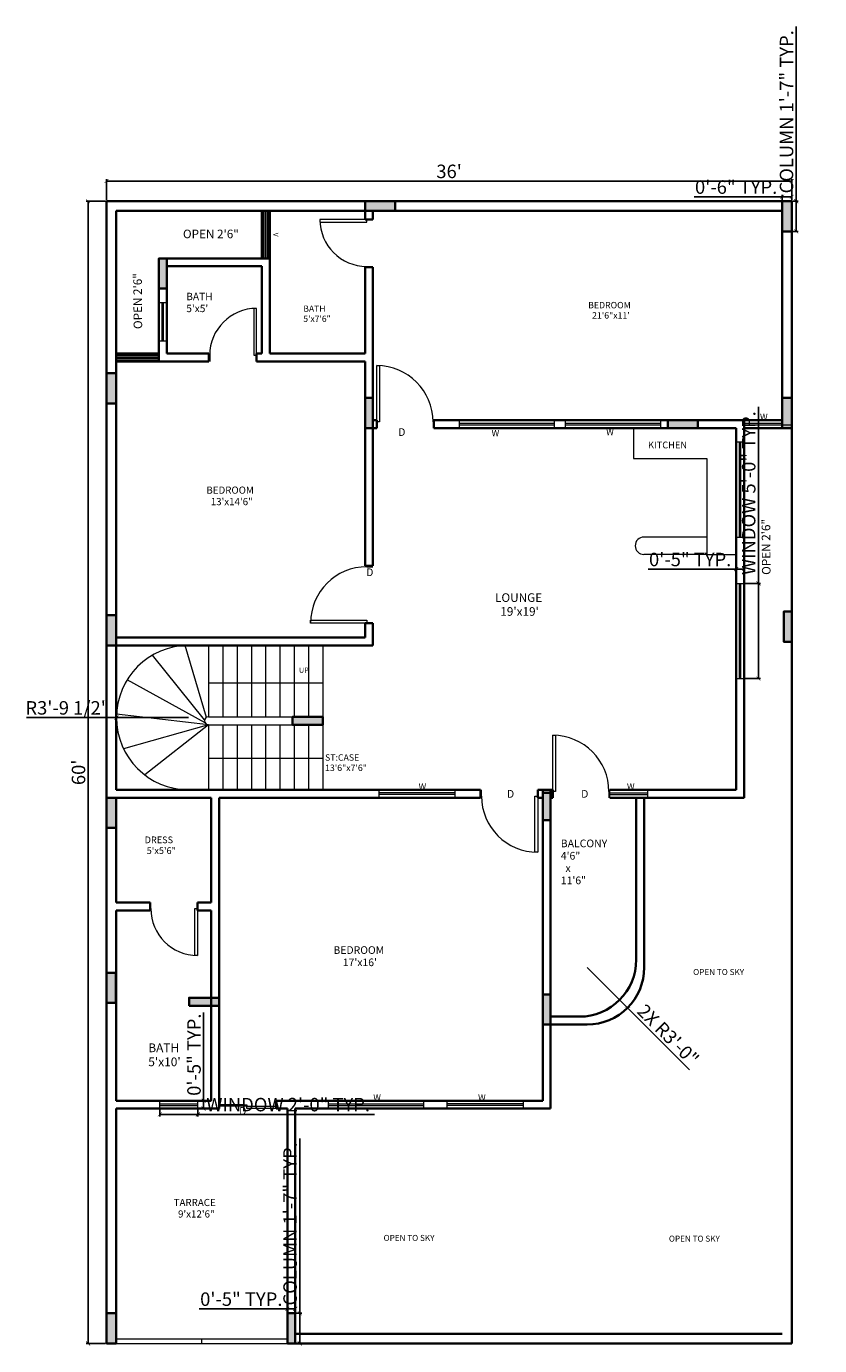
# Model space of a CAD drawing. Units: inches. Extents: x 3799 to 20199, y 1682 to 8087.
# Tile 23 of 30: x 13824 to 14325, y 7134 to 7966. Entities that reach past the tile are written whole.
import ezdxf

# ---------------------------------------------------------------- set-up
doc = ezdxf.new("R2010")
doc.units = ezdxf.units.IN
for name, color, linetype, lineweight in [('A-ANNO-DIMS', 2, 'Continuous', 18), ('A-ANNO-SYMB', 3, 'Continuous', 18), ('A-AREA-IDEN', 7, 'Continuous', 18), ('A-COLS', 251, 'Continuous', 35), ('A-DOOR', 3, 'Continuous', 18), ('A-FLOR-CASE', 32, 'Continuous', 18), ('A-FLOR-RAIL', 217, 'Continuous', 18), ('A-FLOR-STRS', 41, 'Continuous', 18), ('A-GLAZ', 152, 'Continuous', 18), ('A-WALL', 7, 'Continuous', 35)]:
    doc.layers.add(name, color=color, linetype=linetype, lineweight=lineweight)
doc.styles.get("Standard").update_dxf_attribs({"font": 'arial.ttf'})
doc.dimstyles.new('ISO-25', dxfattribs={"dimtxt": 8.5, "dimasz": 2.5, "dimexe": 1.25, "dimexo": 0.625, "dimtad": 1, "dimdec": 0, "dimlunit": 3, "dimtxsty": 'Standard', "dimblk": 'ARCHTICK', "dimcen": 2.5, "dimadec": 0, "dimazin": 0, "dimtfac": 1, "dimtdec": 0, "dimtmove": 0, "dimatfit": 3, "dimfxl": 1, "dimarcsym": 0})

# ---------------------------------------------------------------- blocks, each defined once
blk = doc.blocks.new('*U49')
for p, q in [((0, 0), (0, -100)), ((900, 0), (900, -100))]:
    blk.add_line(p, q)
blk.add_lwpolyline([(0, 0), (0, 900), (43.75, 900), (43.75, 0)], close=True)
blk.add_arc((0, 0), 900, 0, 90)
blk = doc.blocks.new('*U148')
for p, q in [((-750, 0), (-750, -100)), ((0, 0), (0, -100))]:
    blk.add_line(p, q)
blk.add_lwpolyline([(0, 0), (0, 750), (-43.75, 750), (-43.75, 0)], close=True)
blk.add_arc((0, 0), 750, 90, 180)
blk = doc.blocks.new('*U150')
for p, q in [((-900, 0), (-900, 100)), ((0, 0), (0, 100))]:
    blk.add_line(p, q)
blk.add_lwpolyline([(0, 0), (0, -900), (-43.75, -900), (-43.75, 0)], close=True)
blk.add_arc((0, 0), 900, 180, 270)
blk = doc.blocks.new('*U151')
for p, q in [((-750, 0), (-750, 100)), ((0, 0), (0, 100))]:
    blk.add_line(p, q)
blk.add_lwpolyline([(0, 0), (0, -750), (-43.75, -750), (-43.75, 0)], close=True)
blk.add_arc((0, 0), 750, 180, 270)
blk = doc.blocks.new('_ArchTick')
at = {"color": 0, "linetype": 'ByBlock', "const_width": 0.15}
blk.add_lwpolyline([(-0.5, -0.5), (0.5, 0.5)], dxfattribs=at)
blk = doc.blocks.new('*D154')
at = {"layer": 'A-ANNO-DIMS', "color": 0, "lineweight": -2, "transparency": 16777216}
for p, q in [((13875, 7856.48), (13875, 7869.85)), ((13875, 7868.6), (14307, 7868.6)), ((14307, 7856.48), (14307, 7869.85))]:
    blk.add_line(p, q, dxfattribs=at)
at = {"layer": 'Defpoints', "color": 0, "transparency": 16777216}
for p in [(14307, 7868.6), (13875, 7855.85), (14307, 7855.85)]:
    blk.add_point(p, dxfattribs=at)
at = {"layer": 'A-ANNO-DIMS', "color": 0, "lineweight": -2, "transparency": 16777216, "xscale": 2.5, "yscale": 2.5, "zscale": 2.5, "rotation": 180}
blk.add_blockref('_ArchTick', (13875, 7868.6), dxfattribs=at)
at = {"layer": 'A-ANNO-DIMS', "color": 0, "lineweight": -2, "transparency": 16777216, "xscale": 2.5, "yscale": 2.5, "zscale": 2.5}
blk.add_blockref('_ArchTick', (14307, 7868.6), dxfattribs=at)
at = {"layer": 'A-ANNO-DIMS', "color": 0, "transparency": 16777216, "insert": (14091, 7873.57), "char_height": 8.5, "attachment_point": 5}
blk.add_mtext("36'", dxfattribs=at)
blk = doc.blocks.new('*D155')
at = {"layer": 'A-ANNO-DIMS', "color": 0, "lineweight": -2, "transparency": 16777216}
for p, q in [((13874.38, 7855.85), (13862.14, 7855.85)), ((13863.39, 7135.85), (13863.39, 7855.85)), ((13874.38, 7135.85), (13862.14, 7135.85))]:
    blk.add_line(p, q, dxfattribs=at)
at = {"layer": 'Defpoints', "color": 0, "transparency": 16777216}
for p in [(13863.39, 7855.85), (13875, 7855.85), (13875, 7135.85)]:
    blk.add_point(p, dxfattribs=at)
at = {"layer": 'A-ANNO-DIMS', "color": 0, "lineweight": -2, "transparency": 16777216, "xscale": 2.5, "yscale": 2.5, "zscale": 2.5}
for p, rotation in [((13863.39, 7855.85), 90), ((13863.39, 7135.85), 270)]:
    blk.add_blockref('_ArchTick', p, dxfattribs=dict(at, rotation=rotation))
at = {"layer": 'A-ANNO-DIMS', "color": 0, "transparency": 16777216, "insert": (13858.43, 7495.85), "char_height": 8.5, "attachment_point": 5, "rotation": 90}
blk.add_mtext("60'", dxfattribs=at)
blk = doc.blocks.new('WIN-48IN-5IN-FRAME')
for p, q in [((0, 5), (0, 0)), ((48, 3), (0, 3)), ((48, 2), (0, 2)), ((48, 5), (48, 0))]:
    blk.add_line(p, q)
blk = doc.blocks.new('WIN-60IN-5IN-FRAME')
for p, q in [((0, 5), (0, 0)), ((0, 3), (60, 3)), ((0, 2), (60, 2)), ((60, 5), (60, 0))]:
    blk.add_line(p, q)
blk = doc.blocks.new('WIN-24IN-5IN-FRAME')
for p, q in [((0, 0), (0, 5)), ((0, 3), (24, 3)), ((0, 2), (24, 2)), ((24, 0), (24, 5))]:
    blk.add_line(p, q)
blk = doc.blocks.new('COL-6X19IN')
h = blk.add_hatch(color=256)
h.dxf.hatch_style = 1
h.paths.add_polyline_path([(19, 0), (19, 6), (0, 6), (0, 0)])
blk.add_lwpolyline([(0, 0), (19, 0), (19, 6), (0, 6)], close=True)
blk = doc.blocks.new('COL-5X19IN')
h = blk.add_hatch(color=256)
h.dxf.hatch_style = 1
h.paths.add_polyline_path([(19, 0), (19, 5), (0, 5), (0, 0)])
blk.add_lwpolyline([(0, 0), (19, 0), (19, 5), (0, 5)], close=True)
blk = doc.blocks.new('*D272')
at = {"layer": 'A-ANNO-DIMS', "color": 0, "lineweight": -2, "transparency": 16777216}
for p, q in [((13996.85, 7154.85), (13996.85, 7265.07)), ((13994.63, 7154.85), (13998.1, 7154.85)), ((13996.85, 7135.85), (13996.85, 7154.85)), ((13994.63, 7135.85), (13998.1, 7135.85))]:
    blk.add_line(p, q, dxfattribs=at)
at = {"layer": 'Defpoints', "color": 0, "transparency": 16777216}
for p in [(13994, 7154.85), (13996.85, 7154.85), (13994, 7135.85)]:
    blk.add_point(p, dxfattribs=at)
at = {"layer": 'A-ANNO-DIMS', "color": 0, "lineweight": -2, "transparency": 16777216, "xscale": 2.5, "yscale": 2.5, "zscale": 2.5}
for p, rotation in [((13996.85, 7154.85), 90), ((13996.85, 7135.85), 270)]:
    blk.add_blockref('_ArchTick', p, dxfattribs=dict(at, rotation=rotation))
at = {"layer": 'A-ANNO-DIMS', "color": 0, "transparency": 16777216, "insert": (13991.83, 7211.21), "char_height": 8.5, "attachment_point": 5, "rotation": 90}
blk.add_mtext('COLUMN 1\'-7" TYP.', dxfattribs=at)
blk = doc.blocks.new('*D273')
at = {"layer": 'A-ANNO-DIMS', "color": 0, "lineweight": -2, "transparency": 16777216}
for p, q in [((13989, 7157.7), (13933.44, 7157.7)), ((13989, 7155.48), (13989, 7158.95)), ((13994, 7157.7), (13989, 7157.7)), ((13994, 7155.48), (13994, 7158.95))]:
    blk.add_line(p, q, dxfattribs=at)
at = {"layer": 'Defpoints', "color": 0, "transparency": 16777216}
for p in [(13989, 7157.7), (13989, 7154.85), (13994, 7154.85)]:
    blk.add_point(p, dxfattribs=at)
at = {"layer": 'A-ANNO-DIMS', "color": 0, "lineweight": -2, "transparency": 16777216, "xscale": 2.5, "yscale": 2.5, "zscale": 2.5, "rotation": 180}
blk.add_blockref('_ArchTick', (13989, 7157.7), dxfattribs=at)
at = {"layer": 'A-ANNO-DIMS', "color": 0, "lineweight": -2, "transparency": 16777216, "xscale": 2.5, "yscale": 2.5, "zscale": 2.5}
blk.add_blockref('_ArchTick', (13994, 7157.7), dxfattribs=at)
at = {"layer": 'A-ANNO-DIMS', "color": 0, "transparency": 16777216, "insert": (13959.97, 7162.67), "char_height": 8.5, "attachment_point": 5}
blk.add_mtext('0\'-5" TYP.', dxfattribs=at)
blk = doc.blocks.new('*D284')
at = {"layer": 'A-ANNO-DIMS', "color": 0, "lineweight": -2, "transparency": 16777216}
for p, q in [((14309.85, 7855.85), (14309.85, 7966.07)), ((14307.63, 7855.85), (14311.1, 7855.85)), ((14309.85, 7836.85), (14309.85, 7855.85)), ((14307.63, 7836.85), (14311.1, 7836.85))]:
    blk.add_line(p, q, dxfattribs=at)
at = {"layer": 'Defpoints', "color": 0, "transparency": 16777216}
for p in [(14307, 7855.85), (14309.85, 7855.85), (14307, 7836.85)]:
    blk.add_point(p, dxfattribs=at)
at = {"layer": 'A-ANNO-DIMS', "color": 0, "lineweight": -2, "transparency": 16777216, "xscale": 2.5, "yscale": 2.5, "zscale": 2.5}
for p, rotation in [((14309.85, 7855.85), 90), ((14309.85, 7836.85), 270)]:
    blk.add_blockref('_ArchTick', p, dxfattribs=dict(at, rotation=rotation))
at = {"layer": 'A-ANNO-DIMS', "color": 0, "transparency": 16777216, "insert": (14304.83, 7912.21), "char_height": 8.5, "attachment_point": 5, "rotation": 90}
blk.add_mtext('COLUMN 1\'-7" TYP.', dxfattribs=at)
blk = doc.blocks.new('*D285')
at = {"layer": 'A-ANNO-DIMS', "color": 0, "lineweight": -2, "transparency": 16777216}
for p, q in [((14301, 7858.7), (14245.44, 7858.7)), ((14301, 7856.48), (14301, 7859.95)), ((14307, 7858.7), (14301, 7858.7)), ((14307, 7856.48), (14307, 7859.95))]:
    blk.add_line(p, q, dxfattribs=at)
at = {"layer": 'Defpoints', "color": 0, "transparency": 16777216}
for p in [(14301, 7858.7), (14301, 7855.85), (14307, 7855.85)]:
    blk.add_point(p, dxfattribs=at)
at = {"layer": 'A-ANNO-DIMS', "color": 0, "lineweight": -2, "transparency": 16777216, "xscale": 2.5, "yscale": 2.5, "zscale": 2.5, "rotation": 180}
blk.add_blockref('_ArchTick', (14301, 7858.7), dxfattribs=at)
at = {"layer": 'A-ANNO-DIMS', "color": 0, "lineweight": -2, "transparency": 16777216, "xscale": 2.5, "yscale": 2.5, "zscale": 2.5}
blk.add_blockref('_ArchTick', (14307, 7858.7), dxfattribs=at)
at = {"layer": 'A-ANNO-DIMS', "color": 0, "transparency": 16777216, "insert": (14271.97, 7863.67), "char_height": 8.5, "attachment_point": 5}
blk.add_mtext('0\'-6" TYP.', dxfattribs=at)
blk = doc.blocks.new('*D312')
at = {"layer": 'A-ANNO-DIMS', "color": 0, "lineweight": -2, "transparency": 16777216}
for p, q in [((14286, 7614.95), (14286, 7726.26)), ((14277.63, 7614.95), (14287.25, 7614.95)), ((14286, 7554.95), (14286, 7614.95)), ((14277.63, 7554.95), (14287.25, 7554.95))]:
    blk.add_line(p, q, dxfattribs=at)
at = {"layer": 'Defpoints', "color": 0, "transparency": 16777216}
for p in [(14277, 7614.95), (14286, 7614.95), (14277, 7554.95)]:
    blk.add_point(p, dxfattribs=at)
at = {"layer": 'A-ANNO-DIMS', "color": 0, "lineweight": -2, "transparency": 16777216, "xscale": 2.5, "yscale": 2.5, "zscale": 2.5}
for p, rotation in [((14286, 7614.95), 90), ((14286, 7554.95), 270)]:
    blk.add_blockref('_ArchTick', p, dxfattribs=dict(at, rotation=rotation))
at = {"layer": 'A-ANNO-DIMS', "color": 0, "transparency": 16777216, "insert": (14280.98, 7671.86), "char_height": 8.5, "attachment_point": 5, "rotation": 90}
blk.add_mtext('WINDOW 5\'-0" TYP.', dxfattribs=at)
blk = doc.blocks.new('*D313')
at = {"layer": 'A-ANNO-DIMS', "color": 0, "lineweight": -2, "transparency": 16777216}
for p, q in [((14272, 7623.95), (14216.44, 7623.95)), ((14272, 7615.58), (14272, 7625.2)), ((14277, 7623.95), (14272, 7623.95)), ((14277, 7615.58), (14277, 7625.2))]:
    blk.add_line(p, q, dxfattribs=at)
at = {"layer": 'Defpoints', "color": 0, "transparency": 16777216}
for p in [(14272, 7623.95), (14272, 7614.95), (14277, 7614.95)]:
    blk.add_point(p, dxfattribs=at)
at = {"layer": 'A-ANNO-DIMS', "color": 0, "lineweight": -2, "transparency": 16777216, "xscale": 2.5, "yscale": 2.5, "zscale": 2.5, "rotation": 180}
blk.add_blockref('_ArchTick', (14272, 7623.95), dxfattribs=at)
at = {"layer": 'A-ANNO-DIMS', "color": 0, "lineweight": -2, "transparency": 16777216, "xscale": 2.5, "yscale": 2.5, "zscale": 2.5}
blk.add_blockref('_ArchTick', (14277, 7623.95), dxfattribs=at)
at = {"layer": 'A-ANNO-DIMS', "color": 0, "transparency": 16777216, "insert": (14242.97, 7628.92), "char_height": 8.5, "attachment_point": 5}
blk.add_mtext('0\'-5" TYP.', dxfattribs=at)
blk = doc.blocks.new('*D326')
at = {"layer": 'A-ANNO-DIMS', "color": 0, "lineweight": -2, "transparency": 16777216}
for p, q in [((13908.62, 7283.23), (13908.62, 7279)), ((13908.62, 7280.25), (13932.62, 7280.25)), ((13932.62, 7283.23), (13932.62, 7279)), ((13932.62, 7280.25), (14043.93, 7280.25))]:
    blk.add_line(p, q, dxfattribs=at)
at = {"layer": 'Defpoints', "color": 0, "transparency": 16777216}
for p in [(13908.62, 7283.85), (13932.62, 7283.85), (13932.62, 7280.25)]:
    blk.add_point(p, dxfattribs=at)
at = {"layer": 'A-ANNO-DIMS', "color": 0, "lineweight": -2, "transparency": 16777216, "xscale": 2.5, "yscale": 2.5, "zscale": 2.5, "rotation": 180}
blk.add_blockref('_ArchTick', (13908.62, 7280.25), dxfattribs=at)
at = {"layer": 'A-ANNO-DIMS', "color": 0, "lineweight": -2, "transparency": 16777216, "xscale": 2.5, "yscale": 2.5, "zscale": 2.5}
blk.add_blockref('_ArchTick', (13932.62, 7280.25), dxfattribs=at)
at = {"layer": 'A-ANNO-DIMS', "color": 0, "transparency": 16777216, "insert": (13989.53, 7285.28), "char_height": 8.5, "attachment_point": 5}
blk.add_mtext('WINDOW 2\'-0" TYP.', dxfattribs=at)
blk = doc.blocks.new('*D327')
at = {"layer": 'A-ANNO-DIMS', "color": 0, "lineweight": -2, "transparency": 16777216}
for p, q in [((13936.22, 7288.85), (13936.22, 7344.41)), ((13933.25, 7288.85), (13937.47, 7288.85)), ((13936.22, 7283.85), (13936.22, 7288.85)), ((13933.25, 7283.85), (13937.47, 7283.85))]:
    blk.add_line(p, q, dxfattribs=at)
at = {"layer": 'Defpoints', "color": 0, "transparency": 16777216}
for p in [(13932.62, 7288.85), (13936.22, 7288.85), (13932.62, 7283.85)]:
    blk.add_point(p, dxfattribs=at)
at = {"layer": 'A-ANNO-DIMS', "color": 0, "lineweight": -2, "transparency": 16777216, "xscale": 2.5, "yscale": 2.5, "zscale": 2.5}
for p, rotation in [((13936.22, 7288.85), 90), ((13936.22, 7283.85), 270)]:
    blk.add_blockref('_ArchTick', p, dxfattribs=dict(at, rotation=rotation))
at = {"layer": 'A-ANNO-DIMS', "color": 0, "transparency": 16777216, "insert": (13931.26, 7317.88), "char_height": 8.5, "attachment_point": 5, "rotation": 90}
blk.add_mtext('0\'-5" TYP.', dxfattribs=at)
blk = doc.blocks.new('*D388')
at = {"layer": 'A-ANNO-DIMS', "color": 0, "lineweight": -2, "transparency": 16777216}
for p in [(13824.47, 7530.35), (13926.75, 7530.35)]:
    blk.add_line(p, (13881.25, 7530.35), dxfattribs=at)
at = {"layer": 'Defpoints', "color": 0, "transparency": 16777216}
for p in [(13881.25, 7530.35), (13926.75, 7530.35)]:
    blk.add_point(p, dxfattribs=at)
at = {"layer": 'A-ANNO-DIMS', "color": 0, "lineweight": -2, "transparency": 16777216, "xscale": 2.5, "yscale": 2.5, "zscale": 2.5, "rotation": 359.9995504484994}
blk.add_blockref('_ArchTick', (13881.25, 7530.35), dxfattribs=at)
at = {"layer": 'A-ANNO-DIMS', "color": 0, "transparency": 16777216, "insert": (13850.36, 7535.38), "char_height": 8.5, "attachment_point": 5, "rotation": 359.99955}
blk.add_mtext('R3\'-9 1/2"', dxfattribs=at)
blk = doc.blocks.new('*D389')
at = {"layer": 'A-ANNO-DIMS', "color": 0, "lineweight": -2, "transparency": 16777216}
for p in [(14178, 7372.85), (14242.62, 7308.23)]:
    blk.add_line(p, (14203.46, 7347.4), dxfattribs=at)
at = {"layer": 'Defpoints', "color": 0, "transparency": 16777216}
for p in [(14178, 7372.85), (14203.46, 7347.4)]:
    blk.add_point(p, dxfattribs=at)
at = {"layer": 'A-ANNO-DIMS', "color": 0, "lineweight": -2, "transparency": 16777216, "xscale": 2.5, "yscale": 2.5, "zscale": 2.5, "rotation": 135.0003016059661}
blk.add_blockref('_ArchTick', (14203.46, 7347.4), dxfattribs=at)
at = {"layer": 'A-ANNO-DIMS', "color": 0, "transparency": 16777216, "insert": (14228.32, 7329.56), "char_height": 8.5, "attachment_point": 5, "rotation": 315.0003}
blk.add_mtext('2X R3\'-0"', dxfattribs=at)

msp = doc.modelspace()

# ---------------------------------------------------------------- linework, layer by layer
at = {"layer": 'A-DOOR'}
for p, q in [((13962.08, 7286.31), (13946, 7286.31)), ((13962.08, 7285.31), (13946, 7285.31)), ((13963.56, 7285.31), (13961.97, 7285.31)), ((13962.08, 7286.31), (13963.56, 7286.31)), ((13963.56, 7286.31), (13963.56, 7285.31)), ((13963.56, 7283.85), (13963.56, 7285.31)), ((13963.56, 7285.31), (13982, 7285.31)), ((13982, 7283.85), (13963.56, 7283.85))]:
    msp.add_line(p, q, dxfattribs=at)
at = {"layer": 'A-FLOR-CASE'}
for p, q in [((14207.35, 7712.85), (14207.35, 7693.6)), ((14207.35, 7693.6), (14253.47, 7693.6)), ((14253.47, 7693.6), (14253.47, 7633.17)), ((14253.47, 7644.17), (14213.81, 7644.17)), ((14253.47, 7633.17), (14213.81, 7633.17)), ((14253.47, 7633.17), (14272, 7633.17))]:
    msp.add_line(p, q, dxfattribs=at)
msp.add_arc((14213.81, 7638.67), 5.5, 90, 270, dxfattribs=at)
at = {"layer": 'A-FLOR-RAIL'}
for p, q in [((13881, 7138.85), (13989, 7138.85)), ((13881, 7135.85), (13989, 7135.85)), ((13934.86, 7138.85), (13934.86, 7135.85))]:
    msp.add_line(p, q, dxfattribs=at)
at = {"layer": 'A-FLOR-STRS'}
for p, q in [((13936.87, 7528.89), (13904.02, 7569.77)), ((13937.96, 7530.45), (13924.6, 7575.8)), ((13939.31, 7575.85), (13939.31, 7530.85)), ((13948.31, 7575.85), (13948.31, 7530.85)), ((13957.31, 7575.85), (13957.31, 7530.85)), ((13966.31, 7575.85), (13966.31, 7530.85)), ((13975.31, 7575.85), (13975.31, 7530.85)), ((13984.31, 7575.85), (13984.31, 7530.85)), ((13993.31, 7575.85), (13993.31, 7530.85)), ((14002.31, 7575.85), (14002.31, 7530.85)), ((14011.31, 7575.85), (14011.31, 7484.85)), ((13937.2, 7527.02), (13887.96, 7554.13)), ((14011.31, 7552.09), (13939.31, 7552.09)), ((13881, 7530.85), (13881.25, 7530.85)), ((13939.31, 7525.85), (13881.3, 7532.43)), ((13939.31, 7530.85), (14011.31, 7530.85)), ((13881, 7525.85), (13881.48, 7525.85)), ((13939.31, 7525.85), (13885.76, 7510.6)), ((13939.31, 7525.85), (13899.16, 7494.18)), ((13939.31, 7525.85), (14011.31, 7525.85)), ((13939.31, 7525.85), (13939.31, 7484.85)), ((13948.31, 7525.85), (13948.31, 7484.85)), ((13957.31, 7525.85), (13957.31, 7484.85)), ((13966.31, 7525.85), (13966.31, 7484.85)), ((13975.31, 7525.85), (13975.31, 7484.85)), ((13984.31, 7525.85), (13984.31, 7484.85)), ((13993.31, 7525.85), (13993.31, 7484.85)), ((14002.31, 7525.85), (14002.31, 7484.85)), ((13939.31, 7504.79), (14011.31, 7504.79))]:
    msp.add_line(p, q, dxfattribs=at)
for centre, radius in [((13926.75, 7530.35), 45.5), ((13939.31, 7528.35), 2.5)]:
    msp.add_arc(centre, radius, 90, 270, dxfattribs=at)
at = {"layer": 'A-GLAZ'}
for p, q in [((13974, 7849.85), (13974, 7819.85)), ((13975, 7849.85), (13975, 7819.85)), ((13976, 7849.85), (13976, 7819.85)), ((13977, 7849.85), (13977, 7819.85)), ((13881, 7758.85), (13908, 7758.85)), ((13881, 7757.85), (13908, 7757.85)), ((13881, 7756.85), (13908, 7756.85)), ((13881, 7755.85), (13908, 7755.85)), ((14277, 7715.85), (14301, 7715.85)), ((14277, 7714.85), (14307, 7714.85))]:
    msp.add_line(p, q, dxfattribs=at)
at = {"layer": 'A-WALL'}
for p, q in [((13875, 7855.85), (14307, 7855.85)), ((13875, 7135.85), (13875, 7855.85)), ((14307, 7855.85), (14307, 7135.85)), ((13881, 7849.85), (14038, 7849.85)), ((13881, 7580.85), (13881, 7849.85)), ((13973, 7849.85), (13973, 7819.85)), ((13978, 7849.85), (13978, 7759.85)), ((14038, 7849.85), (14038, 7844.33)), ((14038, 7844.33), (14043, 7844.33)), ((14043, 7849.85), (14043, 7844.33)), ((14043, 7849.85), (14301, 7849.85)), ((14301, 7849.85), (14301, 7717.85)), ((13908, 7819.85), (13908, 7754.85)), ((13908, 7819.85), (13978, 7819.85)), ((13913, 7814.85), (13913, 7759.85)), ((13913, 7814.85), (13973, 7814.85)), ((13973, 7814.85), (13973, 7759.85)), ((14038, 7814.33), (14043, 7814.33)), ((14038, 7814.33), (14038, 7759.85)), ((14043, 7814.33), (14043, 7717.85)), ((13881, 7759.85), (13908, 7759.85)), ((13913, 7759.85), (13939.56, 7759.85)), ((13939.56, 7759.85), (13939.56, 7754.85)), ((13969.56, 7759.85), (13969.56, 7754.85)), ((13969.56, 7759.85), (13973, 7759.85)), ((13978, 7759.85), (14038, 7759.85)), ((13881, 7754.85), (13939.56, 7754.85)), ((13969.56, 7754.85), (14038, 7754.85)), ((14038, 7754.85), (14038, 7625.98)), ((14043, 7717.85), (14045.41, 7717.85)), ((14045.41, 7717.85), (14045.41, 7712.85)), ((14081.41, 7717.85), (14081.41, 7712.85)), ((14081.41, 7717.85), (14301, 7717.85)), ((14277, 7717.85), (14277, 7479.85)), ((14043, 7712.85), (14045.41, 7712.85)), ((14043, 7712.85), (14043, 7625.98)), ((14081.41, 7712.85), (14272, 7712.85)), ((14272, 7712.85), (14272, 7484.85)), ((14277, 7712.85), (14307, 7712.85)), ((14038, 7625.98), (14043, 7625.98)), ((14038, 7589.98), (14043, 7589.98)), ((14038, 7589.98), (14038, 7580.85)), ((14043, 7589.98), (14043, 7575.85)), ((13881, 7580.85), (14038, 7580.85)), ((13881, 7575.85), (14043, 7575.85)), ((13881, 7484.85), (13881, 7575.85)), ((13881, 7484.85), (14110.86, 7484.85)), ((14110.86, 7484.85), (14110.86, 7479.85)), ((14146.86, 7484.85), (14146.86, 7479.85)), ((14146.86, 7484.85), (14156.32, 7484.85)), ((14156.32, 7479.85), (14156.32, 7484.85)), ((14192.32, 7484.85), (14272, 7484.85)), ((13881, 7479.85), (13941, 7479.85)), ((13881, 7413.85), (13881, 7479.85)), ((13941, 7413.85), (13941, 7479.85)), ((13946, 7283.85), (13946, 7479.85)), ((13946, 7479.85), (14110.86, 7479.85)), ((14146.86, 7479.85), (14150, 7479.85)), ((14150, 7482.85), (14155, 7482.85)), ((14150, 7288.85), (14150, 7479.85)), ((14155, 7479.85), (14156.32, 7479.85)), ((14155, 7341.85), (14155, 7479.85)), ((14192.32, 7479.85), (14214, 7479.85)), ((14209, 7479.85), (14209, 7377.85)), ((14214, 7479.85), (14277, 7479.85)), ((14214, 7479.85), (14214, 7372.85)), ((13881, 7413.85), (13902.42, 7413.85)), ((13902.42, 7413.85), (13902.42, 7408.85)), ((13932.42, 7413.85), (13932.42, 7408.85)), ((13932.42, 7413.85), (13941, 7413.85)), ((13881, 7408.85), (13902.42, 7408.85)), ((13881, 7288.85), (13881, 7408.85)), ((13932.42, 7408.85), (13941, 7408.85)), ((13941, 7288.85), (13941, 7408.85)), ((14155, 7341.85), (14173, 7341.85)), ((14155, 7283.85), (14155, 7336.85)), ((14155, 7336.85), (14178, 7336.85)), ((13881, 7288.85), (13941, 7288.85)), ((13982, 7288.85), (14150, 7288.85)), ((13982, 7283.85), (13982, 7288.85)), ((13881, 7135.85), (13881, 7283.85)), ((13881, 7283.85), (13946, 7283.85)), ((13982, 7283.85), (13989, 7283.85)), ((13989, 7135.85), (13989, 7283.85)), ((13994, 7141.85), (13994, 7283.85)), ((13994, 7283.85), (14155, 7283.85)), ((13881, 7135.85), (13875, 7135.85)), ((14307, 7135.85), (13989, 7135.85)), ((14301, 7141.85), (13994, 7141.85))]:
    msp.add_line(p, q, dxfattribs=at)
for centre in [(14173, 7377.85), (14178, 7372.85)]:
    msp.add_arc(centre, 36, 270, 0, dxfattribs=at)

# ---------------------------------------------------------------- block references
at = {"layer": 'A-COLS'}
for name, p in [('COL-6X19IN', (14038, 7849.85)), ('COL-5X19IN', (14228.8, 7712.85)), ('COL-5X19IN', (13992.29, 7525.85)), ('COL-5X19IN', (13927, 7348.73))]:
    msp.add_blockref(name, p, dxfattribs=at)
at = {"layer": 'A-COLS', "rotation": 90}
for name, p in [('COL-6X19IN', (14307, 7836.85)), ('COL-5X19IN', (13913, 7800.85)), ('COL-6X19IN', (13881, 7728.41)), ('COL-5X19IN', (14043, 7712.85)), ('COL-6X19IN', (14307, 7712.85)), ('COL-6X19IN', (13881, 7575.85)), ('COL-5X19IN', (14307, 7578.15)), ('COL-5X19IN', (14155, 7465.77)), ('COL-6X19IN', (13881, 7460.85)), ('COL-6X19IN', (13880.95, 7350.47)), ('COL-5X19IN', (14155, 7336.85)), ('COL-6X19IN', (13881, 7135.85)), ('COL-5X19IN', (13994, 7135.85))]:
    msp.add_blockref(name, p, dxfattribs=at)
at = {"layer": 'A-DOOR', "xscale": 0.0393700787401575, "yscale": 0.0393700787401575, "zscale": 0.0393700787401575, "rotation": 90}
for name, p in [('*U148', (14039.07, 7844.33)), ('*U49', (14039.07, 7589.98))]:
    msp.add_blockref(name, p, dxfattribs=at)
at = {"layer": 'A-DOOR', "xscale": 0.0393700787401575, "yscale": 0.0393700787401575, "zscale": 0.0393700787401575}
for name, p in [('*U148', (13969.56, 7758.79)), ('*U49', (14045.41, 7716.79)), ('*U49', (14156.32, 7483.79)), ('*U150', (14146.86, 7480.92)), ('*U151', (13932.42, 7409.92))]:
    msp.add_blockref(name, p, dxfattribs=at)
at = {"layer": 'A-GLAZ', "rotation": 90}
for name, p in [('WIN-24IN-5IN-FRAME', (13913, 7767.71)), ('WIN-60IN-5IN-FRAME', (14277, 7644.14)), ('WIN-60IN-5IN-FRAME', (14277, 7554.95))]:
    msp.add_blockref(name, p, dxfattribs=at)
at = {"layer": 'A-GLAZ'}
for name, p in [('WIN-60IN-5IN-FRAME', (14097.31, 7712.85)), ('WIN-60IN-5IN-FRAME', (14164.2, 7712.85)), ('WIN-48IN-5IN-FRAME', (14046.69, 7479.85)), ('WIN-24IN-5IN-FRAME', (14192.32, 7479.85)), ('WIN-24IN-5IN-FRAME', (13908.62, 7283.85)), ('WIN-60IN-5IN-FRAME', (14014.83, 7283.85)), ('WIN-48IN-5IN-FRAME', (14089.62, 7283.85))]:
    msp.add_blockref(name, p, dxfattribs=at)

# ---------------------------------------------------------------- texts
at = {"layer": 'A-ANNO-SYMB'}
for s, height, rotation, p in [('V', 3.18, 270.00194, (13980.22, 7836.03)), ('W', 3.99, 0.00194, (14287.03, 7717.85)), ('D', 4.86, 0.00194, (14058.89, 7707.92)), ('W', 3.99, 0.00194, (14117.81, 7707.68)), ('W', 3.99, 0.00194, (14190.05, 7708.38)), ('D', 4.86, 0.00194, (14038.69, 7619.55)), ('UP', 3.358, 0.00194, (13996.32, 7558.57)), ('W', 3.99, 0.00194, (14071.78, 7484.85)), ('D', 4.86, 0.00194, (14127.47, 7479.85)), ('D', 4.86, 0.00194, (14174.22, 7479.85)), ('W', 3.99, 0.00194, (14203.14, 7484.85)), ('W', 3.99, 0.00194, (14043.2, 7288.85)), ('W', 3.99, 0.00194, (14109.27, 7288.85)), ('D', 4.86, 0.00194, (13958.59, 7279.98))]:
    msp.add_text(s, height=height, rotation=rotation, dxfattribs=at).set_placement(p)
at = {"layer": 'A-AREA-IDEN'}
for s, height, rotation, p in [('OPEN 2\'6"', 5.409, 0.00194, (13923.19, 7832.53)), ('OPEN 2\'6"', 5.409, 90.40024, (13897.5, 7775.3)), ('BATH', 4.683, 0.00194, (13925.29, 7793.46)), ('BEDROOM', 4.044, 0.00194, (14178.67, 7788.35)), ("5'x5'", 4.683, 0.00194, (13925.29, 7785.94)), ('5\'x7\'6"', 3.96, 0.00194, (13999.07, 7779.8)), ('BATH', 3.96, 0.00194, (13999.07, 7786.16)), ('  21\'6"x11\'', 4.0442, 0.00194, (14178.67, 7781.86)), ('KITCHEN', 4.277, 0.00194, (14216.42, 7700.06)), ('BEDROOM', 4.509, 0.00194, (13937.95, 7671.49)), ('  13\'x14\'6"', 4.5094, 0.00194, (13937.95, 7664.25)), ('OPEN 2\'6"', 5.409, 90.40024, (14293.68, 7620.35)), ('LOUNGE', 5.444, 0.00194, (14119.94, 7603.28)), ("  19'x19'", 5.444, 0.00194, (14119.94, 7594.53)), ('ST:CASE', 4.049, 0.00194, (14012.77, 7503.18)), ('13\'6"x7\'6"', 4.049, 0.00194, (14012.77, 7496.68)), ('DRESS', 4.233, 0.00194, (13899.03, 7451.17)), ('BALCONY', 4.836, 0.00194, (14161.41, 7448.62)), (' 5\'x5\'6"', 4.233, 0.00194, (13899.03, 7444.37)), ('4\'6"', 4.836, 0.00194, (14161.41, 7440.85)), ('  x', 4.836, 0.00194, (14161.41, 7433.08)), ('11\'6"', 4.836, 0.00194, (14161.41, 7425.32)), ('BEDROOM', 4.813, 0.00194, (14018.1, 7381.41)), ("    17'x16'", 4.8126, 0.00194, (14018.1, 7373.68)), ('OPEN TO SKY', 3.7659, 0.00194, (14244.86, 7368.09)), ('BATH', 5.504, 0.00194, (13901.34, 7319.45)), ("5'x10'", 5.504, 0.00194, (13901.34, 7310.6)), ('TARRACE', 4.508, 0.00194, (13917.33, 7222.44)), ('  9\'x12\'6"', 4.508, 0.00194, (13917.33, 7215.2)), ('OPEN TO SKY', 3.7659, 0.00194, (14049.66, 7200.5)), ('OPEN TO SKY', 3.7659, 0.00194, (14229.57, 7200.01))]:
    msp.add_text(s, height=height, rotation=rotation, dxfattribs=at).set_placement(p)

# ---------------------------------------------------------------- dimensions: what is measured, and where the dimension line sits
at = {"layer": 'A-ANNO-DIMS'}
for base, p1, p2, angle, text, picture, middle in [((14309.85, 7855.85), (14307, 7836.85), (14307, 7855.85), 90, 'COLUMN <> TYP.', '*D284', (14304.83, 7912.21)), ((14301, 7858.7), (14307, 7855.85), (14301, 7855.85), 180, '<> TYP.', '*D285', (14271.97, 7863.67)), ((14286, 7614.95), (14277, 7554.95), (14277, 7614.95), 90, 'WINDOW <> TYP.', '*D312', (14280.98, 7671.86)), ((14272, 7623.95), (14277, 7614.95), (14272, 7614.95), 180, '<> TYP.', '*D313', (14242.97, 7628.92)), ((13936.22, 7288.85), (13932.62, 7283.85), (13932.62, 7288.85), 90, '<> TYP.', '*D327', (13931.26, 7317.88)), ((13996.85, 7154.85), (13994, 7135.85), (13994, 7154.85), 90, 'COLUMN <> TYP.', '*D272', (13991.83, 7211.21)), ((13989, 7157.7), (13994, 7154.85), (13989, 7154.85), 180, '<> TYP.', '*D273', (13959.97, 7162.67))]:
    dim = msp.add_linear_dim(base=base, p1=p1, p2=p2, angle=angle, text=text, dimstyle='ISO-25', override={"dimdec": 1, "dimlfac": 1, "dimrnd": 0, "dimzin": 1, "dimdsep": 46, "dimlunit": 4, "dimfrac": 2}, dxfattribs=at)
    dim.commit()
    dim.dimension.update_dxf_attribs({"geometry": picture, "text_midpoint": middle})
dim = msp.add_linear_dim(base=(14307, 7868.6), p1=(13875, 7855.85), p2=(14307, 7855.85), dimstyle='ISO-25', override={"dimclrd": 0, "dimclre": 0, "dimclrt": 0}, dxfattribs=at)
dim.commit()
dim.dimension.update_dxf_attribs({"geometry": '*D154', "text_midpoint": (14091, 7873.57)})
dim = msp.add_linear_dim(base=(13863.39, 7855.85), p1=(13875, 7135.85), p2=(13875, 7855.85), angle=90, dimstyle='ISO-25', override={"dimclrd": 0, "dimclre": 0, "dimclrt": 0}, dxfattribs=at)
dim.commit()
dim.dimension.update_dxf_attribs({"geometry": '*D155', "text_midpoint": (13858.43, 7495.85)})
dim = msp.add_radius_dim(center=(13926.75, 7530.35), mpoint=(13881.25, 7530.35), dimstyle='ISO-25', override={"dimdec": 1, "dimlfac": 1, "dimrnd": 0, "dimzin": 1, "dimdsep": 46, "dimlunit": 4, "dimfrac": 2}, dxfattribs=at)
dim.commit()
dim.dimension.update_dxf_attribs({"geometry": '*D388', "text_midpoint": (13850.36, 7535.38)})
dim = msp.add_radius_dim(center=(14178, 7372.85), mpoint=(14203.46, 7347.4), text='2X <>', dimstyle='ISO-25', override={"dimdec": 1, "dimlfac": 1, "dimrnd": 0, "dimzin": 1, "dimdsep": 46, "dimlunit": 4, "dimfrac": 2}, dxfattribs=at)
dim.commit()
dim.dimension.update_dxf_attribs({"geometry": '*D389', "text_midpoint": (14228.32, 7329.56)})
dim = msp.add_linear_dim(base=(13932.62, 7280.25), p1=(13908.62, 7283.85), p2=(13932.62, 7283.85), text='WINDOW <> TYP.', dimstyle='ISO-25', override={"dimdec": 1, "dimlfac": 1, "dimrnd": 0, "dimzin": 1, "dimdsep": 46, "dimlunit": 4, "dimfrac": 2}, dxfattribs=at)
dim.commit()
dim.dimension.update_dxf_attribs({"geometry": '*D326', "text_midpoint": (13989.53, 7285.28)})

doc.saveas('drawing.dxf')
